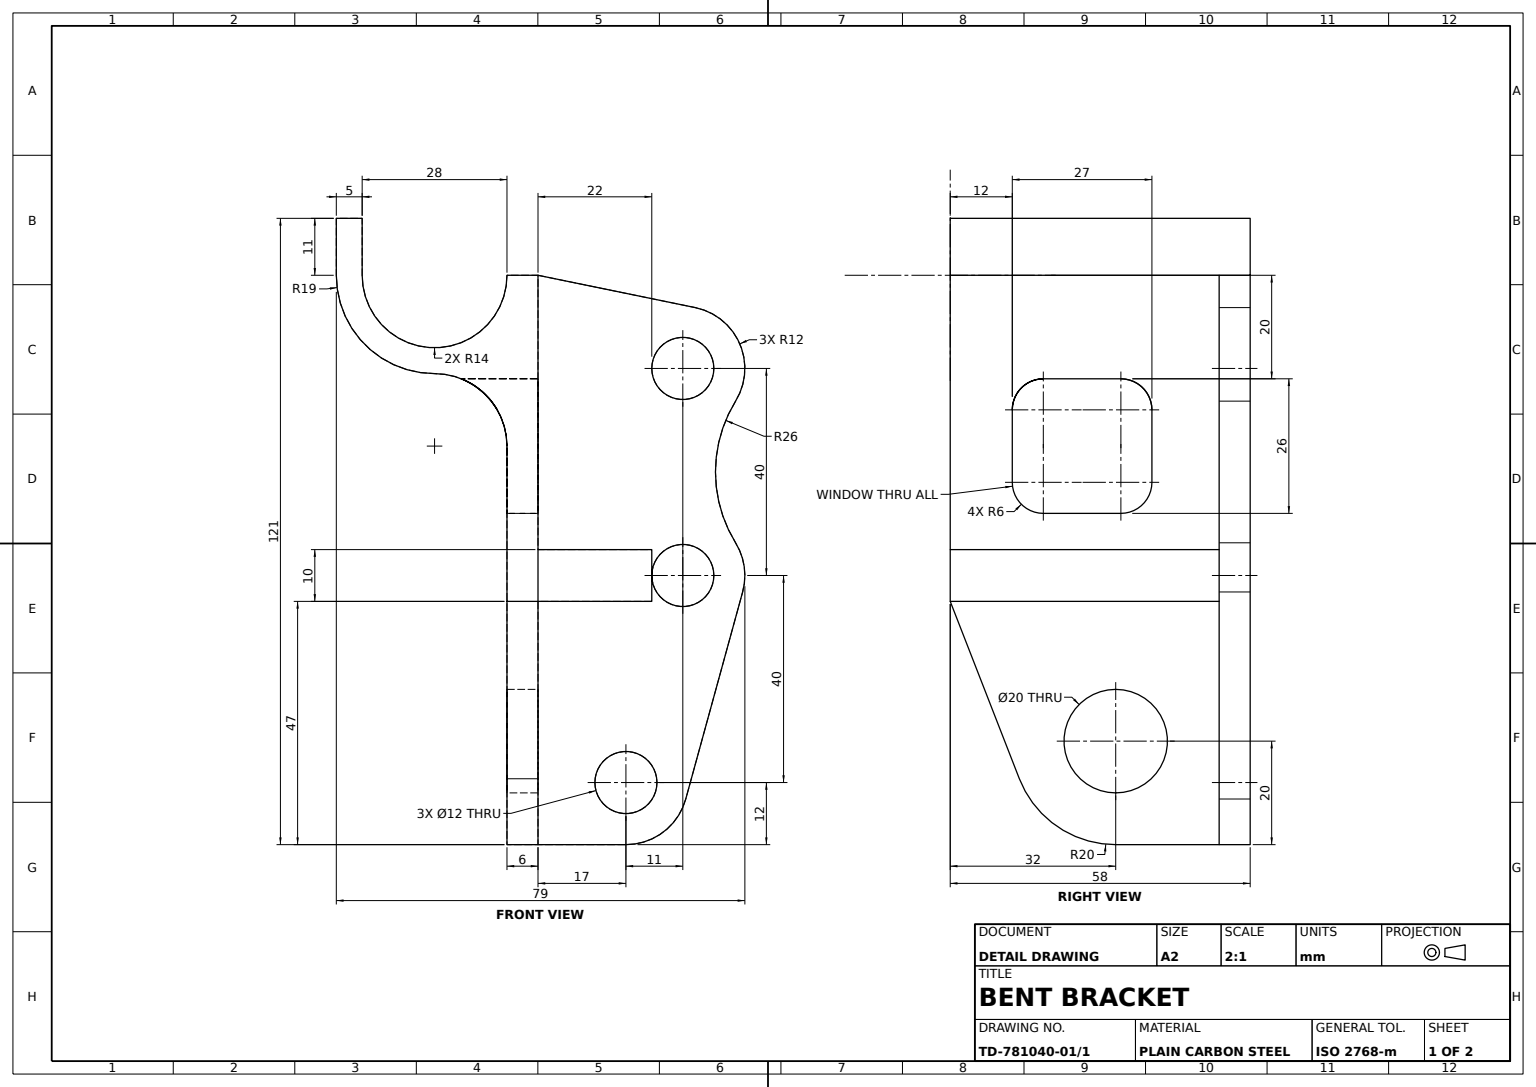
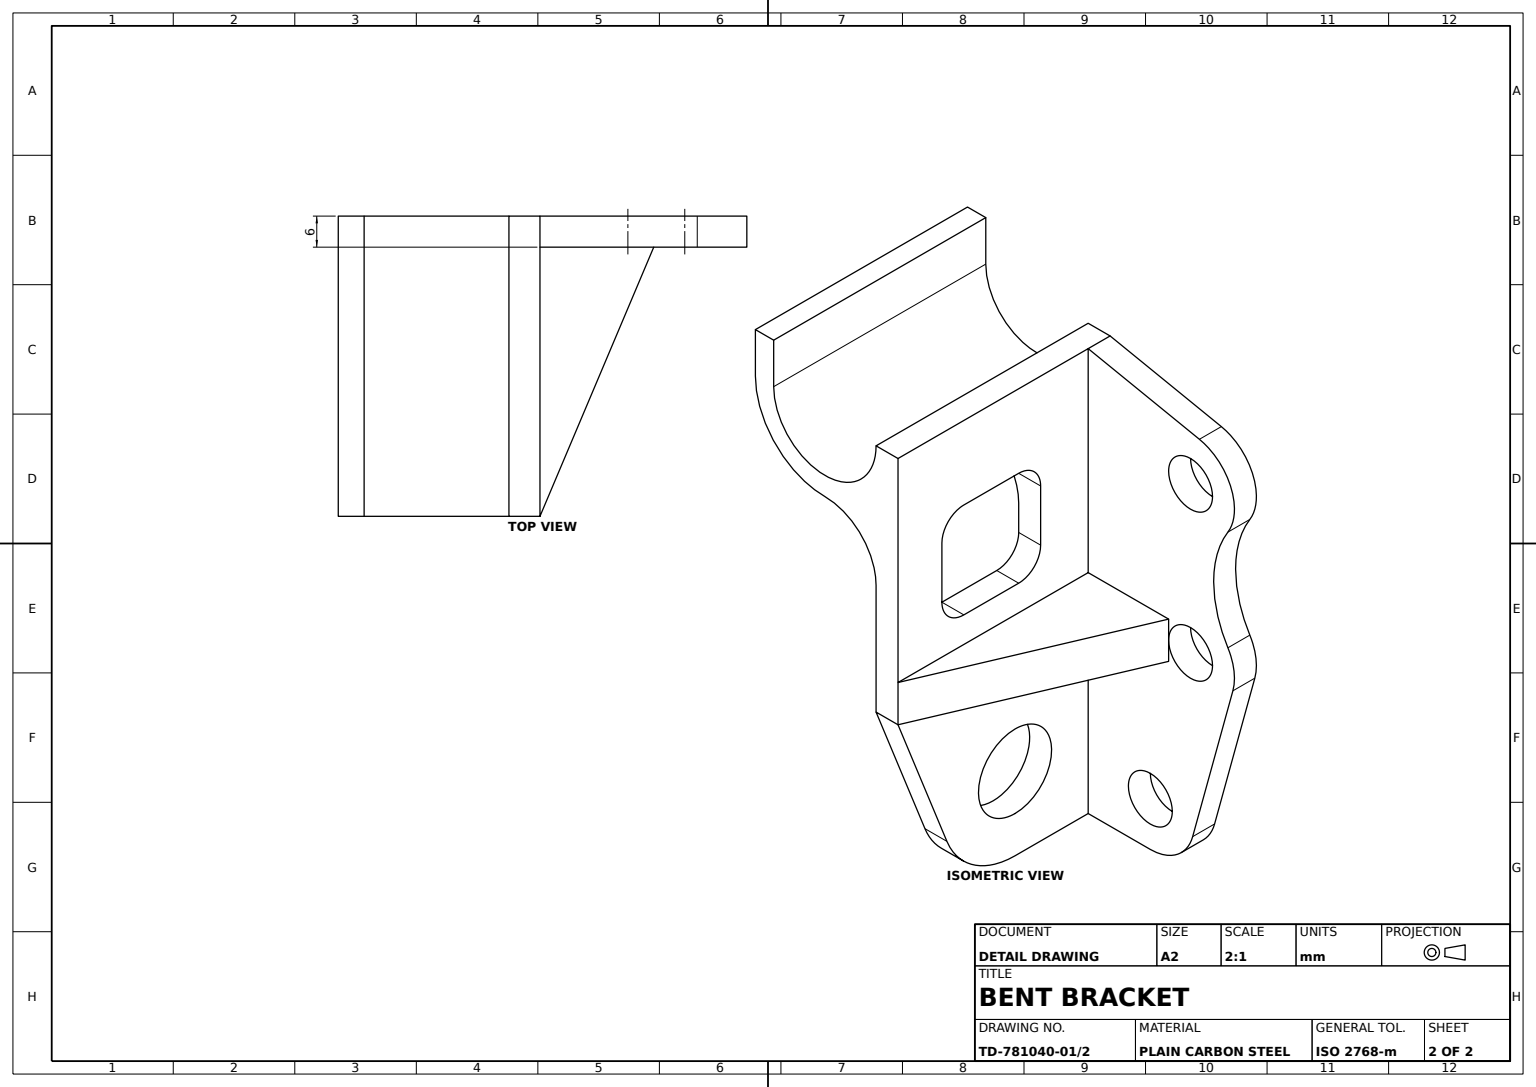
from build123d import *

# Parameters (mm, degrees)
BRACKET_PROFILE_SKETCH_W  = 5
BRACKET_PROFILE_SKETCH_H  = 11
BRACKET_BODY_DEPTH        = 29
SADDLE_START              = -29
SKETCH1_4_R               = 6
SADDLE_STRAP_DEPTH        = 6
SQUARE_WINDOW_20X20_REACH = 86.865
SQUARE_WINDOW_SKETCH_R    = 10
CENTRE_GUSSET_DEPTH       = 5
CORNER_FILLET_R14_R       = 14
EDGE_NOTCH_REACH          = 86.865
EDGE_NOTCH_SKETCH_W       = 27
EDGE_NOTCH_SKETCH_H       = 26
NOTCH_FILLET_R6_R         = 6


with BuildPart() as part:
    # Bracket Profile Sketch → Bracket Body (new, symmetric)
    with BuildSketch(Plane.XY):
        with BuildLine():
            Line((0, -52), (0, 58))
            Line((0, 58), (-6, 58))
            ThreePointArc((-6, 58), (-20, 44), (-34, 58))
            Line((-34, 58), (-39, 58))
            ThreePointArc((-39, 58), (-26.892024376, 40.29406879), (-6, 45.154767421))
            Line((-6, 45.154767421), (-6, -52))
            Line((-6, -52), (0, -52))
        make_face()
        with Locations((-36.5, 63.5)):
            Rectangle(BRACKET_PROFILE_SKETCH_W, BRACKET_PROFILE_SKETCH_H)
    extrude(amount=BRACKET_BODY_DEPTH, both=True)

    # Sketch1_4 → Saddle Strap (add)
    with BuildSketch(Plane.XY.offset(SADDLE_START)):
        with BuildLine():
            ThreePointArc((38.203470161, 33.684210526), (34.310988843, 20), (38.203470161, 6.315789474))
            ThreePointArc((38.203470161, 6.315789474), (39.877604172, 1.709537694), (39.570464714, -3.181877796))
            Line((39.570464714, -3.181877796), (28.570464714, -43.181877796))
            ThreePointArc((28.570464714, -43.181877796), (24.27383896, -49.544174494), (17, -52))
            Line((17, -52), (0, -52))
            Line((0, -52), (0, 58))
            Line((0, 58), (30.413757643, 51.754734112))
            ThreePointArc((30.413757643, 51.754734112), (39.019735252, 44.750308934), (38.203470161, 33.684210526))
        make_face()
        with Locations((28, 40)):
            Circle(SKETCH1_4_R, mode=Mode.SUBTRACT)
        with Locations((28, 0)):
            Circle(SKETCH1_4_R, mode=Mode.SUBTRACT)
        with Locations((17, -40)):
            Circle(SKETCH1_4_R, mode=Mode.SUBTRACT)
    extrude(amount=SADDLE_STRAP_DEPTH)

    # Square Window Sketch → Square Window 20x20 (cut, up to next)
    with BuildSketch(Plane(origin=(0, 0, 0), x_dir=(0, 0, -1), z_dir=(1, 0, 0)), mode=Mode.PRIVATE) as square_window_20x20_sk1:
        with BuildLine():
            ThreePointArc((3, -52), (-8.283512569, -48.513096139), (-15.632572784, -39.268234411))
            Line((-15.632572784, -39.268234411), (-29, -5))
            Line((-29, -5), (-29, -52))
            Line((-29, -52), (3, -52))
        make_face()
    square_window_20x20_tool1 = extrude(square_window_20x20_sk1.sketch, amount=-SQUARE_WINDOW_20X20_REACH, mode=Mode.PRIVATE) & part.part
    # Square Window Sketch → Square Window 20x20 (cut, up to next)
    with BuildSketch(Plane(origin=(0, 0, 0), x_dir=(0, 0, -1), z_dir=(1, 0, 0)), mode=Mode.PRIVATE) as square_window_20x20_sk2:
        with Locations(Location((3, -32, 0), (0, 0, 90))):
            Circle(SQUARE_WINDOW_SKETCH_R)
    square_window_20x20_tool2 = extrude(square_window_20x20_sk2.sketch, amount=-SQUARE_WINDOW_20X20_REACH, mode=Mode.PRIVATE) & part.part
    add(square_window_20x20_tool1.solids().sort_by_distance((0, -37.269178, 21.871829))[0], mode=Mode.SUBTRACT)
    add(square_window_20x20_tool2.solids().sort_by_distance((0, -32, -3))[0], mode=Mode.SUBTRACT)

    # Centre Gusset Sketch → Centre Gusset (add, symmetric)
    with BuildSketch(Plane(origin=(0, 0, 0), x_dir=(1, 0, 0), z_dir=(0, 1, 0))):
        Polygon((0, 23), (0, -29), (22, 23), align=None)
    extrude(amount=CENTRE_GUSSET_DEPTH, both=True)

    # Corner Fillet R14
    corner_fillet_r14_edges = [part.edges().sort_by_distance(p)[0] for p in [
        (-6, 45.154767421, 0),
    ]]
    fillet(corner_fillet_r14_edges, radius=CORNER_FILLET_R14_R)

    # Edge Notch Sketch → Edge Notch (cut, up to next)
    with BuildSketch(Plane(origin=(0, 0, 0), x_dir=(0, 0, -1), z_dir=(1, 0, 0)), mode=Mode.PRIVATE) as edge_notch_sk1:
        with Locations((-3.5, 25)):
            Rectangle(EDGE_NOTCH_SKETCH_W, EDGE_NOTCH_SKETCH_H)
    edge_notch_tool1 = extrude(edge_notch_sk1.sketch, amount=-EDGE_NOTCH_REACH, mode=Mode.PRIVATE) & part.part
    add(edge_notch_tool1.solids().sort_by_distance((0, 25, 3.5))[0], mode=Mode.SUBTRACT)

    # Notch Fillet R6
    notch_fillet_r6_edges = [part.edges().sort_by_distance(p)[0] for p in [
        (-7.401923789, 38, 17),
        (-3, 12, -10),
        (-3, 12, 17),
        (-7.401923789, 38, -10),
    ]]
    fillet(notch_fillet_r6_edges, radius=NOTCH_FILLET_R6_R)


solid = part.part
